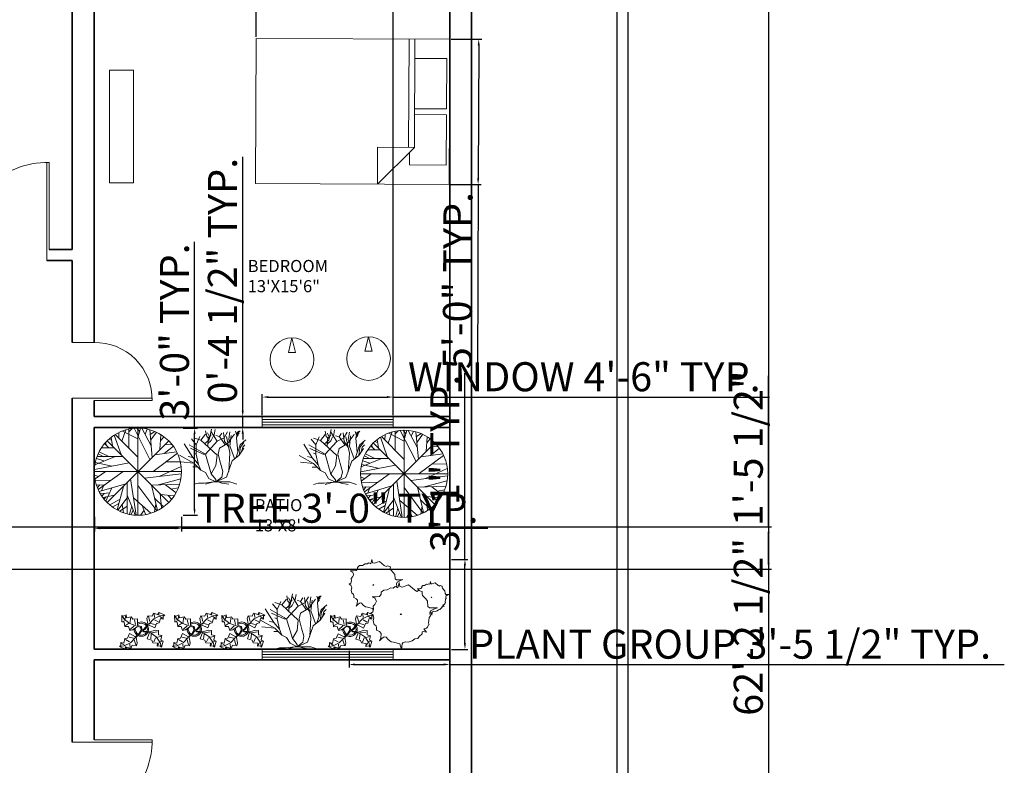
# Model space of a CAD drawing. Units: inches. Extents: x 2562 to 3392, y 1021 to 2243.
# Tile 5 of 6: x 2986 to 3392, y 1665 to 1973. Entities that reach past the tile are written whole.
import ezdxf

# ---------------------------------------------------------------- set-up
doc = ezdxf.new("R2010")
doc.units = ezdxf.units.IN
for name, color, linetype, lineweight in [('A-ANNO-DIMS', 2, 'Continuous', 18), ('A-AREA-IDEN', 7, 'Continuous', 18), ('A-DOOR', 4, 'Continuous', 18), ('A-FURN', 8, 'Continuous', 18), ('A-GLAZ', 4, 'Continuous', 13), ('A-WALL', 7, 'Continuous', 35), ('C-PROP', 7, 'Continuous', 30), ('L-PLNT', 94, 'Continuous', 13), ('M-EQPM', 9, 'Continuous', 18)]:
    doc.layers.add(name, color=color, linetype=linetype, lineweight=lineweight)
doc.styles.get("Standard").update_dxf_attribs({"font": 'arial.ttf'})
doc.dimstyles.new('ISO-25', dxfattribs={"dimtxt": 12, "dimasz": 2.5, "dimexe": 1.25, "dimexo": 0.625, "dimtad": 1, "dimdec": 1, "dimlunit": 3, "dimtxsty": 'Standard', "dimcen": 2.5, "dimadec": 0, "dimazin": 0, "dimtfac": 1, "dimtdec": 1, "dimtmove": 0, "dimatfit": 3, "dimfxl": 1, "dimarcsym": 0})

# ---------------------------------------------------------------- blocks, each defined once
blk = doc.blocks.new('Bed - Queen')
for p, q in [((0, -80.00003), (0, 0)), ((0, 0), (59.99999, 0)), ((59.99999, 0), (59.99999, -80.00003)), ((7.99999, -1.2), (28.79998, -1.2)), ((7.99999, -14.4), (7.99999, -1.2)), ((28.79998, -1.2), (28.79998, -14.4)), ((31.19999, -1.2), (51.99999, -1.2)), ((31.19999, -14.4), (31.19999, -1.2)), ((51.99999, -1.2), (51.99999, -16.4)), ((0, -14.4), (44.8, -14.4)), ((59.99999, -29.6), (44.8, -14.4)), ((44.8, -14.4), (44.8, -29.6)), ((44.8, -16.8), (0, -16.8)), ((51.99999, -16.4), (46.79936, -16.4)), ((44.8, -29.6), (59.99999, -29.6)), ((59.99999, -80.00003), (0, -80.00003))]:
    blk.add_line(p, q)
blk = doc.blocks.new('Compressor')
for p, q in [((0, 0), (-0.05, -0.2)), ((0.05, -0.2), (0, 0)), ((-0.05, -0.2), (0.05, -0.2))]:
    blk.add_line(p, q)
blk.add_circle((0, -0.3), 0.3)
blk = doc.blocks.new('Tree - deciduous plan')
for p, q in [((-22.0458, 42.0753), (-16.5881, 57.6486)), ((-21.1656, 55.8436), (-0.0388, 45.0094)), ((-12.5388, 54.9406), (-7.9613, 59.4546)), ((-12.3627, 32.1443), (-12.5388, 58.7776)), ((-5.3205, 59.6806), (16.5105, 16.7963)), ((2.426, 54.9406), (-1.4472, 59.9056)), ((0, 59.9996), (0, -60)), ((0.4894, 48.6208), (3.6584, 59.6806)), ((18.2711, 35.5298), (5.419, 59.6806)), ((9.8203, 51.5549), (12.8133, 58.5516)), ((19.6795, 19.5047), (16.3344, 57.6486)), ((17.0387, 51.1035), (23.2006, 55.1666)), ((17.7429, 43.6552), (25.4894, 54.2636)), ((42, 42), (-42, -42)), ((42, -42), (-42, 42)), ((-40.1797, 44.558), (-36.4825, 43.2038)), ((-37.0107, 47.0408), (-35.25, 35.5298)), ((-32.6092, 50.4264), (-23.2782, 23.5674)), ((-31.2008, 51.1035), (-0.2149, 20.1818)), ((-26.4472, 46.5894), (-26.2712, 53.8116)), ((31.6513, 50.8778), (30.2429, 30.5643)), ((31.1232, 42.5267), (35.8767, 48.1693)), ((-53.2078, 27.4044), (-40.1797, 20.859)), ((-49.8627, 32.8214), (-32.7853, 32.8214)), ((-45.8134, 38.2383), (-40.5318, 33.0471)), ((-43.8768, 36.4326), (-44.405, 40.2696)), ((23.3767, 23.3417), (53.3063, 27.4044)), ((36.2288, 25.1474), (48.9049, 35.0784)), ((37.1091, 37.1098), (46.6161, 37.5612)), ((-32.2571, 20.6333), (-59.1937, 9.348)), ((-57.081, 17.9248), (-47.0458, 14.7649)), ((-56.0247, 20.859), (-20.8134, 20.859)), ((-54.7923, 24.4702), (-47.75, 21.0847)), ((54.3626, 25.3731), (20.9119, 0.3198)), ((38.5175, 13.4107), (58.2359, 13.6364)), ((-59.7219, 2.8025), (-12.0106, 12.0565)), ((-58.6656, 12.7336), (-35.9543, 7.5424)), ((-54.6162, -24.7335), (-20.2853, 0.0941)), ((29.3626, -6.6771), (59.4682, 7.091)), ((-60, 0), (60, 0)), ((-59.7219, -4.8714), (-54.2641, -6.6771)), ((-45.2853, -0.1316), (-59.0177, -10.0627)), ((-58.4895, -12.3197), (-36.4825, -11.6426)), ((-10.074, -10.0627), (-2.5036, -59.7178)), ((9.2922, -9.1598), (59.6443, -2.8401)), ((26.3697, -18.4138), (58.9401, -9.8369)), ((-57.081, -18.4138), (-45.2853, -17.9624)), ((-52.6797, -18.188), (-55.4966, -22.0251)), ((-53.2078, -27.442), (-16.7641, -16.6081)), ((-47.2219, -19.3166), (-50.2148, -26.3135)), ((-35.9543, -22.4765), (-44.0529, -40.5329)), ((-19.9331, -20.2194), (-28.5599, -52.721)), ((-14.8275, -15.0282), (-14.6515, -57.6865)), ((-0.0388, -19.0909), (25.8415, -53.8495)), ((18.6232, -18.6394), (26.7218, -53.3981)), ((18.7992, -18.6394), (57.3556, -17.2853)), ((38.1654, -18.188), (52.426, -29.0219)), ((45.9119, -24.0564), (55.595, -22.2508)), ((-38.9472, -29.0219), (-51.4472, -30.6018)), ((-46.5177, -30.1504), (-49.5106, -33.536)), ((-32.4331, -32.4075), (-48.1021, -35.5674)), ((-43.7008, -34.6645), (-46.6937, -37.373)), ((-24.6867, -37.8244), (-38.7712, -45.7241)), ((-14.6515, -36.2445), (-27.6797, -52.9467)), ((-14.6515, -32.1818), (-3.912, -59.4922)), ((-6.2008, -36.2445), (17.919, -57.0094)), ((22.8485, -36.4702), (35.3485, -48.4326)), ((30.419, -30.1504), (32.3556, -50.0125)), ((31.4753, -31.279), (49.6091, -33.3103)), ((41.5105, -32.6332), (46.088, -38.0501)), ((-26.2712, -43.9185), (-34.7219, -48.6583)), ((-14.6515, -47.3041), (-25.0388, -54.3009)), ((-21.5177, -45.4984), (-19.9331, -56.1065)), ((-8.4895, -47.5298), (-11.4825, -58.5893)), ((-6.3768, -52.721), (-9.3698, -58.815)), ((8.4119, -53.1724), (3.8344, -59.4922)), ((5.9471, -46.6269), (10.5246, -58.5893)), ((24.7852, -44.8213), (23.0246, -54.978))]:
    blk.add_line(p, q)
blk.add_circle((0, 0), 60)
blk = doc.blocks.new('Clump of Trees or Bushes - plan')
for points in [[(-10.993, 56.487), (-9.228, 58.426), (-10.144, 63.512), (-8.923, 67.033), (-3.43, 69.772), (2.673, 72.119), (-2.82, 71.728), (-10.449, 71.728), (-13.195, 74.075), (-13.806, 83.073), (-16.857, 86.594), (-22.045, 92.071), (-22.961, 94.81), (-22.656, 98.722), (-28.759, 100.678), (-31.811, 99.113), (-35.472, 101.461), (-45.543, 109.676), (-49.815, 108.503), (-55.308, 106.155), (-59.58, 106.938), (-60.801, 113.98), (-63.242, 104.982), (-67.209, 106.938), (-70.872, 104.59), (-74.839, 104.982), (-80.637, 101.461), (-86.435, 101.069), (-90.402, 97.548), (-90.402, 94.419), (-93.454, 90.898), (-98.947, 90.115), (-105.66, 90.115), (-101.083, 87.768), (-98.031, 82.682), (-100.778, 77.596), (-103.829, 74.466), (-103.219, 69.772), (-104.134, 65.077), (-108.102, 62.73), (-104.439, 60.774), (-102.609, 55.297), (-103.829, 50.211), (-102.303, 44.342), (-98.947, 41.995), (-98.031, 38.865), (-98.031, 34.953), (-93.148, 32.606), (-90.707, 29.476), (-91.317, 22.434), (-93.454, 17.348), (-89.487, 21.26), (-85.519, 23.999), (-82.468, 23.216), (-78.806, 19.304), (-74.228, 15.783), (-69.956, 15.392), (-59.886, 12.653), (-58.254, 7.074)], [(59.448, 5.262), (60.936, 4.858), (62.652, -1.011), (63.415, 4.858), (64.178, 5.836), (66.848, 6.814), (69.709, 6.569), (73.905, 7.792), (76.385, 9.748), (79.627, 10.237), (81.153, 12.438), (84.014, 15.127), (84.205, 17.084), (85.158, 17.573), (88.591, 16.839), (85.73, 20.262), (88.591, 20.751), (89.545, 21.974), (90.689, 24.174), (91.452, 24.663), (90.499, 25.886), (91.261, 31.999), (92.596, 33.466), (92.024, 36.645), (92.787, 38.845), (96.22, 40.557), (100.035, 42.024), (96.602, 41.779), (91.834, 41.779), (90.117, 43.246), (89.736, 48.871), (87.828, 51.071), (84.586, 54.494), (84.014, 56.206), (84.205, 58.651), (80.39, 59.873), (78.483, 58.895), (76.194, 60.362), (69.9, 65.497), (67.23, 64.764), (63.797, 63.297), (61.126, 63.786), (60.364, 68.187), (58.838, 62.563), (56.358, 63.786), (54.07, 62.319), (51.59, 62.563), (47.966, 60.362), (44.343, 60.118), (41.863, 57.917), (41.863, 55.961), (39.956, 53.761), (36.523, 53.272), (32.327, 53.272), (35.187, 51.805), (36.641, 49.381)]]:
    blk.add_lwpolyline(points)
for points in [[(-4.577, 66.508), (-7.629, 55.261), (-12.588, 57.706), (-17.166, 54.772), (-22.125, 55.261), (-29.372, 50.86), (-36.62, 50.371), (-41.579, 45.969), (-41.579, 42.057), (-45.393, 37.656), (-52.259, 36.678), (-60.651, 36.678), (-54.93, 33.743), (-51.115, 27.386), (-54.548, 21.029), (-58.363, 17.116), (-57.6, 11.248), (-58.744, 5.38), (-63.703, 2.446), (-59.126, 0), (-56.837, -6.846), (-58.363, -13.203), (-56.455, -20.539), (-52.259, -23.473), (-51.115, -27.385), (-51.115, -32.275), (-45.012, -35.21), (-41.96, -39.122), (-42.723, -47.924), (-45.393, -54.282), (-40.434, -49.391), (-35.475, -45.968), (-31.661, -46.946), (-27.083, -51.837), (-21.362, -56.238), (-16.021, -56.727), (-3.433, -60.15), (0, -71.887), (1.526, -60.15), (3.052, -58.194), (8.392, -56.238), (14.114, -56.727), (22.506, -54.282), (27.465, -50.369), (33.949, -49.391), (37.001, -44.99), (42.723, -39.611), (43.104, -35.699), (45.012, -34.721), (51.878, -36.188), (46.156, -29.341), (51.878, -28.363), (53.785, -25.918), (56.074, -21.517), (57.6, -20.539), (55.692, -18.094), (57.218, -5.868), (59.888, -2.934), (58.744, 3.424), (60.27, 7.825), (67.136, 11.248), (74.765, 14.182), (67.899, 13.693), (58.363, 13.693), (54.93, 16.627), (54.167, 27.875), (50.352, 32.276), (43.867, 39.123), (42.723, 42.546), (43.104, 47.436), (35.475, 49.882), (31.661, 47.925), (27.083, 50.86), (14.495, 61.129), (9.155, 59.662), (2.289, 56.728), (-3.052, 57.706)], [(-58.055, 61.947), (-58.97, 60.774), (-57.139, 60.774)], [(62.08, 35.667), (61.508, 34.933), (62.652, 34.933)], [(-1.144, 1.468), (-2.289, 0), (0, 0)]]:
    blk.add_lwpolyline(points, close=True)
blk = doc.blocks.new('Shrub - elevation')
for p, q in [((-14.88, 18.24), (-12.96, 20.64)), ((-12.471, 19.775), (-12.898, 22.044)), ((-11.28, 19.619), (-12.104, 21.184)), ((-11.921, 18.836), (-10.64, 20.401)), ((-11.433, 18.289), (-10.457, 22.749)), ((-8.16, 17.76), (-10.56, 21.6)), ((-9.48, 19.775), (-8.992, 22.592)), ((-7.2, 19.68), (-6.24, 21.12)), ((-5.086, 17.741), (-5.513, 21.34)), ((-5.28, 19.2), (-3.84, 21.6)), ((-3.84, 16.8), (-0.96, 20.64)), ((-3.377, 18.602), (-2.888, 21.575)), ((-0.508, 21.888), (-0.081, 20.558)), ((-0.203, 19.149), (0.102, 21.34)), ((-0.142, 19.384), (0.59, 20.401)), ((-0.02, 20.01), (0.896, 21.105)), ((0.041, 20.714), (1.384, 22.044)), ((0.102, 21.34), (0.835, 21.888)), ((-18.24, 11.04), (-21.755, 16.655)), ((-12.96, 12.48), (-19.68, 16.32)), ((-16.8, 16.32), (-18.72, 18.72)), ((-14.88, 18.24), (-17.76, 19.2)), ((-16.8, 16.32), (-15.36, 19.68)), ((-16.8, 12.48), (-16.8, 16.32)), ((-8.16, 12), (-14.88, 18.24)), ((-13.325, 16.724), (-11.433, 18.289)), ((-12.96, 12.48), (-8.16, 17.76)), ((-11.677, 19.071), (-12.471, 19.775)), ((-12.043, 15.628), (-11.921, 18.836)), ((-11.982, 16.802), (-10.579, 18.054)), ((-10.579, 18.054), (-9.846, 19.697)), ((-7.2, 19.68), (-8.64, 20.16)), ((-8.16, 17.76), (-5.28, 19.2)), ((-4.8, 16.32), (-7.2, 19.68)), ((-7.2, 14.88), (-3.84, 16.8)), ((-3.377, 15.315), (-5.086, 17.819)), ((-2.88, 12.96), (-4.32, 19.68)), ((-2.766, 16.802), (-3.377, 18.602)), ((-2.88, 15.84), (-2.4, 20.16)), ((0.346, 13.203), (-0.203, 19.149)), ((1.323, 16.254), (3.642, 18.289)), ((1.44, 15.36), (2.88, 17.28)), ((2.4, 15.36), (3.36, 16.32)), ((-13.92, 12.48), (-19.2, 14.88)), ((-16.8, 12.48), (-17.76, 12.96)), ((-15.84, 8.16), (-16.8, 12.48)), ((-12.96, 12.48), (-13.92, 12.48)), ((-10.56, 4.32), (-12.96, 12.48)), ((-7.68, 12.48), (-7.2, 14.88)), ((-6.72, 8.64), (-7.68, 12.48)), ((-3.36, 5.28), (-2.88, 12.96)), ((-0.96, 10.56), (-2.88, 15.84)), ((-0.48, 10.8), (0.346, 13.203)), ((0.346, 13.203), (1.323, 16.254)), ((0.96, 12), (1.44, 15.36)), ((0.96, 12), (2.88, 14.88)), ((1.92, 13.44), (2.4, 15.36)), ((-17.76, 8.64), (-23.663, 11.961)), ((-17.76, 8.64), (-23.128, 9.222)), ((-18.24, 11.04), (-20.16, 11.52)), ((-15.84, 8.16), (-18.24, 11.04)), ((-14.88, 5.76), (-17.76, 8.64)), ((-14.88, 5.76), (-15.84, 8.16)), ((-8.64, 7.68), (-8.16, 12)), ((-5.76, 5.28), (-6.72, 8.64)), ((-4.32, 2.88), (-1.92, 9.6)), ((-1.92, 9.6), (0.96, 12)), ((-16.32, 7.2), (-18.24, 7.2)), ((-12.96, 4.8), (-14.88, 5.76)), ((-11.52, 2.4), (-12.96, 4.8)), ((-10.56, 4.32), (-8.64, 7.68)), ((-8.64, 1.92), (-10.56, 4.32)), ((-6.24, 2.88), (-5.76, 5.28)), ((-15.84, 0.48), (-17.76, 0)), ((-13.44, 0.48), (-15.84, 0.48)), ((-9.6, 0.96), (-13.44, 0.48)), ((-9.6, 0.96), (-12.96, 0)), ((-8.64, 0.96), (-11.52, 2.4)), ((-9.6, 0.96), (-7.68, 0.96)), ((-8.64, 0.96), (-4.32, 2.88)), ((-8.64, 0.96), (-6.24, 2.88)), ((-8.64, 0.96), (-8.64, 1.92)), ((-8.64, 0.96), (-2.88, 0.96)), ((-7.68, 0.96), (-6.24, 0.48)), ((-6.24, 0.48), (-3.36, 0)), ((-2.88, 0.96), (0, 0))]:
    blk.add_line(p, q)
blk = doc.blocks.new('Plant - Rubber or Philodendron')
for p, q in [((-16.2005, 11.4774), (-13.9899, 8.1064)), ((-16.2005, 11.4774), (-14.8639, 10.7964)), ((-16.0159, 6.3329), (-16.2005, 11.4774)), ((-14.8639, 10.7964), (-12.6195, 11.8975)), ((-13.3174, 8.325), (-13.0735, 11.0065)), ((-12.6195, 11.8975), (-12.1909, 9.4345)), ((-12.1909, 9.4345), (-8.3829, 10.3)), ((-8.8369, 9.409), (-9.0894, 5.6095)), ((-8.3829, 10.3), (-7.0549, 8.501)), ((-7.0549, 8.501), (-3.0284, 8.6941)), ((-3.0284, 8.6941), (-3.0709, 3.1041)), ((4.6914, 8.8812), (5.3859, 11.2828)), ((4.6914, 8.8812), (5.5014, 4.4831)), ((5.3859, 11.2828), (8.8871, 10.7908)), ((5.9878, 10.4842), (7.1971, 6.3869)), ((10.3916, 8.7942), (6.2847, 4.4028)), ((8.8871, 10.7908), (9.9809, 13.4933)), ((9.9809, 13.4933), (13.3837, 12.301)), ((15.3859, 11.3055), (10.3916, 8.7942)), ((10.5828, 12.6946), (10.8893, 9.7953)), ((13.3837, 12.301), (14.68, 13.9039)), ((14.5816, 13.2037), (14.3848, 11.8033)), ((14.68, 13.9039), (19.3848, 11.8146)), ((15.7909, 9.1065), (14.8995, 5.3044)), ((15.2875, 10.6053), (17.5907, 9.2105)), ((19.3848, 11.8146), (15.3859, 11.3055)), ((18.1925, 8.4119), (15.7909, 9.1065)), ((19.3848, 11.8146), (18.1868, 10.9119)), ((18.1868, 10.9119), (18.1925, 8.4119)), ((-14.0069, 5.8704), (-16.0159, 6.3329)), ((-15.3434, 6.5514), (-13.9984, 6.9884)), ((-13.5868, 2.2894), (-14.0069, 5.8704)), ((-13.9899, 8.1064), (-9.5434, 4.7185)), ((-10.6784, 2.491), (-13.5868, 2.2894)), ((-13.1329, 3.1804), (-10.6614, 4.727)), ((-9.5858, -0.8715), (-10.6784, 2.491)), ((-9.5434, 4.7185), (-4.1917, 2.9888)), ((-9.1318, 0.0195), (-5.9793, 2.9025)), ((-7.1228, -0.443), (-3.5248, 2.2131)), ((-4.8529, 4.012), (-5.7184, 7.82)), ((-3.5248, 2.2131), (-3.3011, 2.4355)), ((-3.3011, 2.4355), (-0.5306, 1.7947)), ((-3.0709, 3.1041), (0.0797, 2.3163)), ((-0.5306, 1.7947), (-0.2255, -0.5527)), ((-0.5306, 1.7947), (-0.5306, 1.7947)), ((0.0797, 2.3163), (0.4866, -0.031)), ((0.4866, -0.031), (2.1141, 0.2298)), ((2.1141, 0.2298), (5.4346, 3.9146)), ((6.1032, 3.6844), (2.8262, -0.031)), ((5.4346, 3.9146), (5.5014, 4.4831)), ((11.1089, 1.1958), (6.1032, 3.6844)), ((7.7005, 4.8881), (11.5025, 3.9967)), ((14.2977, 6.1031), (10.9934, 7.9956)), ((12.7005, 4.8994), (11.1089, 1.1958)), ((14.8995, 5.3044), (12.7005, 4.8994)), ((-14.4141, -11.4699), (-13.5228, -7.6679)), ((-13.5228, -7.6679), (-11.3237, -7.2629)), ((-11.3237, -7.2629), (-9.7321, -3.5593)), ((-6.3237, -7.2516), (-10.1257, -6.3602)), ((-9.7321, -3.5593), (-4.7264, -6.0479)), ((-7.1228, -0.443), (-9.5858, -0.8715)), ((-9.0148, -11.1577), (-4.9047, -6.8122)), ((-2.019, -3.6148), (-4.7264, -6.0479)), ((-4.1246, -6.8466), (-4.0579, -6.2781)), ((-3.3146, -11.2447), (-4.1246, -6.8466)), ((-4.0579, -6.2781), (-0.9375, -3.1608)), ((-2.019, -3.6148), (-0.2255, -0.5527)), ((-0.9375, -3.1608), (0.5883, -0.8135)), ((0.5883, -0.8135), (2.2447, -2.0916)), ((2.8262, -0.031), (1.3003, -0.5527)), ((1.3003, -0.5527), (2.4193, -1.4655)), ((2.2447, -2.0916), (6.7108, -2.6626)), ((2.4193, -1.4655), (6.895, -2.1175)), ((4.943, -7.9659), (6.7108, -2.6626)), ((8.8321, -9.0266), (4.943, -7.9659)), ((11.6605, -0.5413), (6.895, -2.1175)), ((12.3677, -6.1981), (7.219, -2.6772)), ((8.125, -4.0768), (7.7715, -7.9659)), ((8.3544, -2.7453), (13.1973, -2.1704)), ((10.2463, -10.4408), (11.6605, -6.9053)), ((11.6605, -0.5413), (14.1354, -0.8948)), ((15.5496, -10.7943), (12.3677, -6.1981)), ((16.2567, -5.8446), (13.4283, -6.5517)), ((14.1354, -0.8948), (14.1354, -4.4304)), ((14.1354, -4.4304), (16.9638, -5.1375)), ((16.9638, -5.1375), (16.2567, -8.673)), ((-18.008, -14.1781), (-16.8101, -13.2754)), ((-18.008, -14.1781), (-14.0091, -13.669)), ((-13.3032, -16.2674), (-18.008, -14.1781)), ((-16.8157, -10.7754), (-14.4141, -11.4699)), ((-16.8101, -13.2754), (-16.8157, -10.7754)), ((-13.9107, -12.9688), (-16.2139, -11.574)), ((-14.0091, -13.669), (-9.0148, -11.1577)), ((-12.0069, -14.6645), (-13.3032, -16.2674)), ((-13.2048, -15.5672), (-13.008, -14.1668)), ((-12.921, -8.4665), (-9.6166, -10.359)), ((-8.6042, -15.8568), (-12.0069, -14.6645)), ((-9.206, -15.0581), (-9.5126, -12.1588)), ((-7.5103, -13.1543), (-8.6042, -15.8568)), ((-4.0092, -13.6463), (-7.5103, -13.1543)), ((-4.611, -12.8477), (-5.8203, -8.7504)), ((-3.3146, -11.2447), (-4.0092, -13.6463)), ((9.5392, -11.1479), (8.8321, -9.0266)), ((13.4283, -11.5015), (9.5392, -11.1479)), ((13.0748, -13.9763), (13.4283, -11.5015)), ((15.5496, -13.6228), (13.0748, -13.9763)), ((14.8425, -10.7943), (13.7819, -13.2692)), ((16.6103, -14.6834), (15.5496, -10.7943)), ((16.6103, -14.6834), (15.5496, -13.6228)), ((17.3174, -9.7337), (15.9032, -9.7337)), ((16.2567, -8.673), (18.0245, -9.7337)), ((18.0245, -9.7337), (16.6103, -14.6834))]:
    blk.add_line(p, q)
for centre, radius, start, end in [((0.0308, 0.1664), 6, 178.6147, 235.1169), ((0.0308, 0.1664), 5, 168.1647, 238.6725), ((0, 0), 6.1275, 34.37569, 120.1028), ((-0.0601, -0.2075), 5.2461, 33.82192, 124.9414), ((-0.2664, 0.1682), 5.2775, 338.4094, 20.03007), ((-0.098, 0.1364), 6.1288, 341.2017, 26.09184), ((-0.0234, 0.3825), 6.1492, 242.5812, 331.2714), ((-0.1102, 0.4886), 5.2883, 247.3711, 327.472)]:
    blk.add_arc(centre, radius, start, end)
blk = doc.blocks.new('Window - Wood Frame 36 in. Wide plan')
for p, q in [((0, 6), (0, 0)), ((36, 6), (36, 0)), ((0, 4.5), (36, 4.5)), ((0, 3), (36, 3)), ((0, 1.5), (36, 1.5))]:
    blk.add_line(p, q)
blk = doc.blocks.new('*D29')
at = {"layer": 'A-ANNO-DIMS', "color": 0, "lineweight": -2, "transparency": 16777216}
for p, q in [((3085.79, 1809.76), (3085.79, 1818.48)), ((3139.79, 1809.76), (3139.79, 1818.48)), ((3088.29, 1817.23), (3137.29, 1817.23)), ((3139.79, 1817.23), (3295.39, 1817.23))]:
    blk.add_line(p, q, dxfattribs=at)
at = {"layer": 'A-ANNO-DIMS', "color": 0, "transparency": 16777216}
for points in [[(3088.29, 1817.65), (3088.29, 1816.82), (3085.79, 1817.23)], [(3137.29, 1817.65), (3137.29, 1816.82), (3139.79, 1817.23)]]:
    blk.add_solid(points, dxfattribs=at)
at = {"layer": 'Defpoints', "color": 0, "transparency": 16777216}
for p in [(3139.79, 1817.23), (3085.79, 1809.13), (3139.79, 1809.13)]:
    blk.add_point(p, dxfattribs=at)
at = {"layer": 'A-ANNO-DIMS', "color": 0, "transparency": 16777216, "insert": (3218.84, 1824.07), "char_height": 12, "attachment_point": 5}
blk.add_mtext('WINDOW 4\'-6" TYP.', dxfattribs=at)
blk = doc.blocks.new('*D30')
at = {"layer": 'A-ANNO-DIMS', "color": 0, "lineweight": -2, "transparency": 16777216}
for p, q in [((3077.69, 1811.63), (3077.69, 1916.49)), ((3085.17, 1809.13), (3076.44, 1809.13)), ((3077.69, 1804.63), (3077.69, 1809.13)), ((3085.17, 1804.63), (3076.44, 1804.63)), ((3077.69, 1802.13), (3077.69, 1799.63))]:
    blk.add_line(p, q, dxfattribs=at)
at = {"layer": 'A-ANNO-DIMS', "color": 0, "transparency": 16777216}
for points in [[(3077.28, 1811.63), (3078.11, 1811.63), (3077.69, 1809.13)], [(3077.28, 1802.13), (3078.11, 1802.13), (3077.69, 1804.63)]]:
    blk.add_solid(points, dxfattribs=at)
at = {"layer": 'Defpoints', "color": 0, "transparency": 16777216}
for p in [(3077.69, 1809.13), (3085.79, 1809.13), (3085.79, 1804.63)]:
    blk.add_point(p, dxfattribs=at)
at = {"layer": 'A-ANNO-DIMS', "color": 0, "transparency": 16777216, "insert": (3070.86, 1865.31), "char_height": 12, "attachment_point": 5, "rotation": 90}
blk.add_mtext('0\'-4 1/2" TYP.', dxfattribs=at)
blk = doc.blocks.new('*D33')
at = {"layer": 'A-ANNO-DIMS', "color": 0, "lineweight": -2, "transparency": 16777216}
for p, q in [((3083.21, 1966.02), (3083.26, 1978.64)), ((3085.76, 1977.38), (3160.76, 1977.07)), ((3163.21, 1965.69), (3163.26, 1978.31)), ((3163.26, 1977.06), (3278.75, 1976.59))]:
    blk.add_line(p, q, dxfattribs=at)
at = {"layer": 'A-ANNO-DIMS', "color": 0, "transparency": 16777216}
for points in [[(3085.76, 1977.8), (3085.76, 1976.97), (3083.26, 1977.39)], [(3160.76, 1977.49), (3160.76, 1976.66), (3163.26, 1977.06)]]:
    blk.add_solid(points, dxfattribs=at)
at = {"layer": 'Defpoints', "color": 0, "transparency": 16777216}
for p in [(3163.26, 1977.06), (3083.21, 1965.4), (3163.21, 1965.06)]:
    blk.add_point(p, dxfattribs=at)
at = {"layer": 'A-ANNO-DIMS', "color": 0, "transparency": 16777216, "insert": (3222.28, 1983.57), "char_height": 12, "attachment_point": 5, "rotation": 359.7633}
blk.add_mtext('BED 6\'-8" TYP.', dxfattribs=at)
blk = doc.blocks.new('*D34')
at = {"layer": 'A-ANNO-DIMS', "color": 0, "lineweight": -2, "transparency": 16777216}
for p, q in [((3163.83, 1965.06), (3176.46, 1965.01)), ((3175.2, 1962.51), (3174.97, 1907.52)), ((3163.59, 1905.06), (3176.21, 1905.01)), ((3174.96, 1905.02), (3174.64, 1828.12))]:
    blk.add_line(p, q, dxfattribs=at)
at = {"layer": 'A-ANNO-DIMS', "color": 0, "transparency": 16777216}
for points in [[(3174.78, 1962.52), (3175.61, 1962.51), (3175.21, 1965.01)], [(3174.55, 1907.52), (3175.39, 1907.51), (3174.96, 1905.02)]]:
    blk.add_solid(points, dxfattribs=at)
at = {"layer": 'Defpoints', "color": 0, "transparency": 16777216}
for p in [(3163.21, 1965.06), (3162.96, 1905.07), (3174.96, 1905.02)]:
    blk.add_point(p, dxfattribs=at)
at = {"layer": 'A-ANNO-DIMS', "color": 0, "transparency": 16777216, "insert": (3168.04, 1865.35), "char_height": 12, "attachment_point": 5, "rotation": 89.7633}
blk.add_mtext('5\'-0" TYP.', dxfattribs=at)
blk = doc.blocks.new('*D53')
at = {"layer": 'A-ANNO-DIMS', "color": 0, "lineweight": -2, "transparency": 16777216}
for p, q in [((3016.41, 1767.78), (3016.41, 1761.76)), ((3052.41, 1767.78), (3052.41, 1761.76)), ((3018.91, 1763.01), (3049.91, 1763.01)), ((3052.41, 1763.01), (3178.98, 1763.01))]:
    blk.add_line(p, q, dxfattribs=at)
at = {"layer": 'A-ANNO-DIMS', "color": 0, "transparency": 16777216}
for points in [[(3018.91, 1763.42), (3018.91, 1762.59), (3016.41, 1763.01)], [(3049.91, 1763.42), (3049.91, 1762.59), (3052.41, 1763.01)]]:
    blk.add_solid(points, dxfattribs=at)
at = {"layer": 'Defpoints', "color": 0, "transparency": 16777216}
for p in [(3016.41, 1768.41), (3052.41, 1768.41), (3052.41, 1763.01)]:
    blk.add_point(p, dxfattribs=at)
at = {"layer": 'A-ANNO-DIMS', "color": 0, "transparency": 16777216, "insert": (3116.94, 1769.76), "char_height": 12, "attachment_point": 5}
blk.add_mtext('TREE 3\'-0" TYP.', dxfattribs=at)
blk = doc.blocks.new('*D54')
at = {"layer": 'A-ANNO-DIMS', "color": 0, "lineweight": -2, "transparency": 16777216}
for p, q in [((3057.81, 1804.41), (3057.81, 1881.29)), ((3053.04, 1804.41), (3059.06, 1804.41)), ((3057.81, 1770.91), (3057.81, 1801.91)), ((3053.04, 1768.41), (3059.06, 1768.41))]:
    blk.add_line(p, q, dxfattribs=at)
at = {"layer": 'A-ANNO-DIMS', "color": 0, "transparency": 16777216}
for points in [[(3057.39, 1801.91), (3058.23, 1801.91), (3057.81, 1804.41)], [(3057.39, 1770.91), (3058.23, 1770.91), (3057.81, 1768.41)]]:
    blk.add_solid(points, dxfattribs=at)
at = {"layer": 'Defpoints', "color": 0, "transparency": 16777216}
for p in [(3052.41, 1804.41), (3057.81, 1804.41), (3052.41, 1768.41)]:
    blk.add_point(p, dxfattribs=at)
at = {"layer": 'A-ANNO-DIMS', "color": 0, "transparency": 16777216, "insert": (3051.05, 1844.1), "char_height": 12, "attachment_point": 5, "rotation": 90}
blk.add_mtext('3\'-0" TYP.', dxfattribs=at)
blk = doc.blocks.new('*D63')
at = {"layer": 'A-ANNO-DIMS', "color": 0, "lineweight": -2, "transparency": 16777216}
for p, q in [((3121.64, 1712.38), (3121.64, 1705.51)), ((3163.27, 1712.38), (3163.27, 1705.51)), ((3124.14, 1706.76), (3160.77, 1706.76)), ((3163.27, 1706.76), (3392.35, 1706.76))]:
    blk.add_line(p, q, dxfattribs=at)
at = {"layer": 'A-ANNO-DIMS', "color": 0, "transparency": 16777216}
for points in [[(3124.14, 1707.18), (3124.14, 1706.34), (3121.64, 1706.76)], [(3160.77, 1707.18), (3160.77, 1706.34), (3163.27, 1706.76)]]:
    blk.add_solid(points, dxfattribs=at)
at = {"layer": 'Defpoints', "color": 0, "transparency": 16777216}
for p in [(3121.64, 1713), (3163.27, 1713), (3163.27, 1706.76)]:
    blk.add_point(p, dxfattribs=at)
at = {"layer": 'A-ANNO-DIMS', "color": 0, "transparency": 16777216, "insert": (3279.06, 1713.6), "char_height": 12, "attachment_point": 5}
blk.add_mtext('PLANT GROUP 3\'-5 1/2" TYP.', dxfattribs=at)
blk = doc.blocks.new('*D64')
at = {"layer": 'A-ANNO-DIMS', "color": 0, "lineweight": -2, "transparency": 16777216}
for p, q in [((3169.51, 1750.18), (3169.51, 1827.06)), ((3163.89, 1750.18), (3170.76, 1750.18)), ((3169.51, 1715.5), (3169.51, 1747.68)), ((3163.89, 1713), (3170.76, 1713))]:
    blk.add_line(p, q, dxfattribs=at)
at = {"layer": 'A-ANNO-DIMS', "color": 0, "transparency": 16777216}
for points in [[(3169.09, 1747.68), (3169.93, 1747.68), (3169.51, 1750.18)], [(3169.09, 1715.5), (3169.93, 1715.5), (3169.51, 1713)]]:
    blk.add_solid(points, dxfattribs=at)
at = {"layer": 'Defpoints', "color": 0, "transparency": 16777216}
for p in [(3163.27, 1750.18), (3169.51, 1750.18), (3163.27, 1713)]:
    blk.add_point(p, dxfattribs=at)
at = {"layer": 'A-ANNO-DIMS', "color": 0, "transparency": 16777216, "insert": (3162.76, 1789.87), "char_height": 12, "attachment_point": 5, "rotation": 90}
blk.add_mtext('3\'-1" TYP.', dxfattribs=at)
blk = doc.blocks.new('*D70')
at = {"layer": 'A-ANNO-DIMS', "color": 0, "lineweight": -2, "transparency": 16777216}
for p, q in [((3172.89, 2095.63), (3296.21, 2095.63)), ((3294.96, 2093.13), (3294.96, 1351.49)), ((3114.84, 1348.99), (3296.21, 1348.99))]:
    blk.add_line(p, q, dxfattribs=at)
at = {"layer": 'A-ANNO-DIMS', "color": 0, "transparency": 16777216}
for points in [[(3294.55, 2093.13), (3295.38, 2093.13), (3294.96, 2095.63)], [(3294.55, 1351.49), (3295.38, 1351.49), (3294.96, 1348.99)]]:
    blk.add_solid(points, dxfattribs=at)
at = {"layer": 'Defpoints', "color": 0, "transparency": 16777216}
for p in [(3172.26, 2095.63), (3114.22, 1348.99), (3294.96, 1348.99)]:
    blk.add_point(p, dxfattribs=at)
at = {"layer": 'A-ANNO-DIMS', "color": 0, "transparency": 16777216, "insert": (3288.13, 1722.31), "char_height": 12, "attachment_point": 5, "rotation": 90}
blk.add_mtext('62\'-2 1/2"', dxfattribs=at)
blk = doc.blocks.new('*D76')
at = {"layer": 'A-ANNO-DIMS', "color": 0, "lineweight": -2, "transparency": 16777216}
for p, q in [((3294.96, 1763.57), (3294.96, 1826.05)), ((2913.39, 1763.57), (3296.21, 1763.57)), ((3294.96, 1748.63), (3294.96, 1761.07)), ((2913.39, 1746.13), (3296.21, 1746.13))]:
    blk.add_line(p, q, dxfattribs=at)
at = {"layer": 'A-ANNO-DIMS', "color": 0, "transparency": 16777216}
for points in [[(3294.55, 1761.07), (3295.38, 1761.07), (3294.96, 1763.57)], [(3294.55, 1748.63), (3295.38, 1748.63), (3294.96, 1746.13)]]:
    blk.add_solid(points, dxfattribs=at)
at = {"layer": 'Defpoints', "color": 0, "transparency": 16777216}
for p in [(2912.76, 1763.57), (3294.96, 1763.57), (2912.76, 1746.13)]:
    blk.add_point(p, dxfattribs=at)
at = {"layer": 'A-ANNO-DIMS', "color": 0, "transparency": 16777216, "insert": (3288.13, 1796.06), "char_height": 12, "attachment_point": 5, "rotation": 90}
blk.add_mtext('1\'-5 1/2"', dxfattribs=at)
blk = doc.blocks.new('*D77')
at = {"layer": 'A-ANNO-DIMS', "color": 0, "lineweight": -2, "transparency": 16777216}
for p, q in [((3139.79, 1809.76), (3139.79, 2219.58)), ((3142.29, 2218.33), (3160.76, 2218.33)), ((3163.26, 1809.76), (3163.26, 2219.58)), ((3163.26, 2218.33), (3235.07, 2218.33))]:
    blk.add_line(p, q, dxfattribs=at)
at = {"layer": 'A-ANNO-DIMS', "color": 0, "transparency": 16777216}
for points in [[(3142.29, 2218.75), (3142.29, 2217.92), (3139.79, 2218.33)], [(3160.76, 2218.75), (3160.76, 2217.92), (3163.26, 2218.33)]]:
    blk.add_solid(points, dxfattribs=at)
at = {"layer": 'Defpoints', "color": 0, "transparency": 16777216}
for p in [(3163.26, 2218.33), (3139.79, 1809.13), (3163.26, 1809.13)]:
    blk.add_point(p, dxfattribs=at)
at = {"layer": 'A-ANNO-DIMS', "color": 0, "transparency": 16777216, "insert": (3200.41, 2225.16), "char_height": 12, "attachment_point": 5}
blk.add_mtext('1\'-11 1/2"', dxfattribs=at)

msp = doc.modelspace()

# ---------------------------------------------------------------- linework, layer by layer
at = {"layer": 'A-DOOR'}
for p, q in [((2997.71, 1914.13), (2996.71, 1914.13)), ((2996.71, 1914.13), (2996.71, 1873.63)), ((2997.71, 1878.13), (2997.71, 1914.13)), ((2996.71, 1873.63), (2997.71, 1873.63)), ((3007.26, 1839.74), (3016.26, 1839.74)), ((3040.26, 1816.74), (3007.26, 1816.74)), ((3016.26, 1815.74), (3040.26, 1815.74)), ((3040.26, 1815.74), (3040.26, 1816.74)), ((3040.26, 1674.7), (3007.26, 1674.7)), ((3016.26, 1675.7), (3040.26, 1675.7)), ((3040.26, 1675.7), (3040.26, 1674.7))]:
    msp.add_line(p, q, dxfattribs=at)
for centre, radius, start, end in [((2997.21, 1878.63), 35.5, 89.1931, 180.8069), ((3016.76, 1816.24), 23.51, 358.7811, 91.2189), ((3007.49, 1675.2), 32.78, 269.6005, 0.8741)]:
    msp.add_arc(centre, radius, start, end, dxfattribs=at)
at = {"layer": 'A-FURN'}
msp.add_lwpolyline([(3022.6, 1952.2), (3032.52, 1952.2), (3032.52, 1905.65), (3022.6, 1905.65)], close=True, dxfattribs=at)
at = {"layer": 'A-WALL'}
for p, q in [((3172.26, 2095.63), (3172.26, 1360.63)), ((3007.26, 2086.63), (3007.26, 1878.13)), ((3163.26, 2086.63), (3163.26, 1365.13)), ((3016.26, 1990.63), (3016.26, 1839.74)), ((2997.71, 1878.13), (3007.26, 1878.13)), ((2996.71, 1873.63), (3007.26, 1873.63)), ((3007.26, 1873.63), (3007.26, 1839.74)), ((3007.26, 1816.74), (3007.26, 1674.7)), ((3016.26, 1815.74), (3016.26, 1809.13)), ((3016.26, 1809.13), (3163.26, 1809.13)), ((3016.26, 1804.63), (3163.26, 1804.63)), ((3016.26, 1804.63), (3016.26, 1713.13)), ((3016.26, 1713.13), (3163.26, 1713.13)), ((3016.26, 1708.63), (3163.26, 1708.63)), ((3016.26, 1708.63), (3016.26, 1675.7))]:
    msp.add_line(p, q, dxfattribs=at)
at = {"layer": 'C-PROP'}
for p, q in [((3236.76, 2160.13), (3236.76, 1080.13)), ((3232.26, 2155.63), (3232.26, 1084.63))]:
    msp.add_line(p, q, dxfattribs=at)

# ---------------------------------------------------------------- block references
at = {"layer": 'A-FURN', "rotation": 269.7632571631042}
msp.add_blockref('Bed - Queen', (3163.21, 1965.06), dxfattribs=at)
at = {"layer": 'A-GLAZ', "xscale": 1.5, "yscale": 0.75}
for p in [(3085.79, 1804.63), (3085.79, 1708.63)]:
    msp.add_blockref('Window - Wood Frame 36 in. Wide plan', p, dxfattribs=at)
at = {"layer": 'L-PLNT'}
for name, p, xscale, yscale in [('Tree - deciduous plan', (3034.41, 1786.41, 1), 0.3, 0.3), ('Tree - deciduous plan', (3144.39, 1785.54, 1), 0.3, 0.3), ('Clump of Trees or Bushes - plan', (3143.26, 1727.38), 0.2, 0.2), ('Plant - Rubber or Philodendron', (3035.79, 1721.27), 0.5, 0.5), ('Plant - Rubber or Philodendron', (3057.67, 1721.27), 0.5, 0.5), ('Plant - Rubber or Philodendron', (3077.21, 1721.27), 0.5, 0.5), ('Plant - Rubber or Philodendron', (3122.01, 1721.23), 0.5, 0.5)]:
    msp.add_blockref(name, p, dxfattribs=dict(at, xscale=xscale, yscale=yscale))
for p in [(3075.28, 1781.22, 1), (3124.68, 1781.11, 1), (3108.77, 1713.13)]:
    msp.add_blockref('Shrub - elevation', p, dxfattribs=at)
at = {"layer": 'M-EQPM', "xscale": 30, "yscale": 30, "zscale": 30}
for p in [(3098.06, 1841.69), (3129.69, 1842.13)]:
    msp.add_blockref('Compressor', p, dxfattribs=at)

# ---------------------------------------------------------------- texts
at = {"layer": 'A-AREA-IDEN', "char_height": 5, "attachment_point": 1}
for s, insert in [('BEDROOM \\P13\'X15\'6"', (3079.77, 1873.86)), ("PATIO \\P13'X8'", (3082.72, 1775.07))]:
    msp.add_mtext(s, dxfattribs=dict(at, insert=insert))

# ---------------------------------------------------------------- dimensions: what is measured, and where the dimension line sits
at = {"layer": 'A-ANNO-DIMS'}
dim = msp.add_linear_dim(base=(3163.26, 2218.33), p1=(3139.79, 1809.13), p2=(3163.26, 1809.13), dimstyle='ISO-25', override={"dimdec": 1, "dimlfac": 1, "dimrnd": 0, "dimzin": 1, "dimdsep": 46, "dimlunit": 4, "dimfrac": 2}, dxfattribs=at)
dim.commit()
dim.dimension.update_dxf_attribs({"geometry": '*D77', "text_midpoint": (3200.41, 2225.16)})
for base, p1, p2, picture, middle in [((3294.96, 1348.99), (3172.26, 2095.63), (3114.22, 1348.99), '*D70', (3288.13, 1722.31)), ((3294.96, 1763.57), (2912.76, 1746.13), (2912.76, 1763.57), '*D76', (3288.13, 1796.06))]:
    dim = msp.add_linear_dim(base=base, p1=p1, p2=p2, angle=90, dimstyle='ISO-25', override={"dimdec": 1, "dimlfac": 1, "dimrnd": 0, "dimzin": 1, "dimdsep": 46, "dimlunit": 4, "dimfrac": 2}, dxfattribs=at)
    dim.commit()
    dim.dimension.update_dxf_attribs({"geometry": picture, "text_midpoint": middle})
for base, p1, p2, angle, text, picture, middle in [((3163.26, 1977.06), (3083.21, 1965.4), (3163.21, 1965.06), 359.7633, 'BED <> TYP.', '*D33', (3222.28, 1983.57)), ((3174.96, 1905.02), (3163.21, 1965.06), (3162.96, 1905.07), 269.7633, '<> TYP.', '*D34', (3168.04, 1865.35)), ((3077.69, 1809.13), (3085.79, 1804.63), (3085.79, 1809.13), 90, '<> TYP.', '*D30', (3070.86, 1865.31)), ((3057.81, 1804.41), (3052.41, 1768.41), (3052.41, 1804.41), 90, '<> TYP.', '*D54', (3051.05, 1844.1)), ((3169.51, 1750.18), (3163.27, 1713), (3163.27, 1750.18), 90, '<> TYP.', '*D64', (3162.76, 1789.87))]:
    dim = msp.add_linear_dim(base=base, p1=p1, p2=p2, angle=angle, text=text, dimstyle='ISO-25', override={"dimdec": 1, "dimlfac": 1, "dimrnd": 0, "dimzin": 1, "dimdsep": 46, "dimlunit": 4, "dimfrac": 2}, dxfattribs=at)
    dim.commit()
    dim.dimension.update_dxf_attribs({"geometry": picture, "text_midpoint": middle})
for base, p1, p2, text, picture, middle in [((3139.79, 1817.23), (3085.79, 1809.13), (3139.79, 1809.13), 'WINDOW <> TYP.', '*D29', (3218.84, 1824.07)), ((3052.41, 1763.01), (3016.41, 1768.41), (3052.41, 1768.41), 'TREE <> TYP.', '*D53', (3116.94, 1769.76)), ((3163.27, 1706.76), (3121.64, 1713), (3163.27, 1713), 'PLANT GROUP <> TYP.', '*D63', (3279.06, 1713.6))]:
    dim = msp.add_linear_dim(base=base, p1=p1, p2=p2, text=text, dimstyle='ISO-25', override={"dimdec": 1, "dimlfac": 1, "dimrnd": 0, "dimzin": 1, "dimdsep": 46, "dimlunit": 4, "dimfrac": 2}, dxfattribs=at)
    dim.commit()
    dim.dimension.update_dxf_attribs({"geometry": picture, "text_midpoint": middle})

doc.saveas('drawing.dxf')
